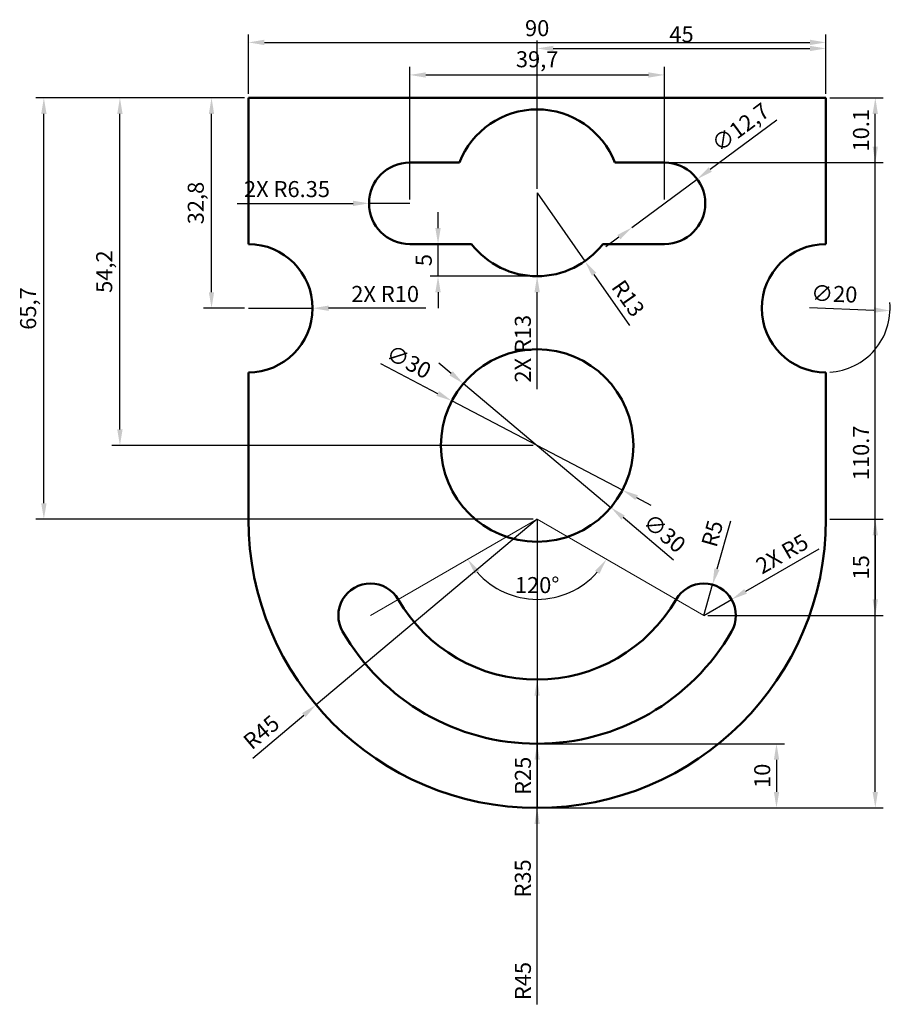
# Model space of a CAD drawing. Units: millimetres. Extents: x 2184 to 2320, y 1849 to 2003.
import ezdxf

# ---------------------------------------------------------------- set-up
doc = ezdxf.new("R2010")
doc.units = ezdxf.units.MM
for name, color, linetype, lineweight in [('M-CONS', 8, 'Continuous', 13), ('M-DIMS', 2, 'Continuous', 25), ('M-OUTL', 7, 'Continuous', 50)]:
    doc.layers.add(name, color=color, linetype=linetype, lineweight=lineweight)
doc.styles.get("Standard").update_dxf_attribs({"font": 'arial.ttf'})
doc.dimstyles.new('ISO-25', dxfattribs={"dimtxt": 2.5, "dimasz": 2.5, "dimexe": 1.25, "dimexo": 0.625, "dimtad": 1, "dimtxsty": 'Standard', "dimcen": 2.5, "dimadec": 0, "dimazin": 0, "dimtfac": 1, "dimtmove": 0, "dimatfit": 3, "dimfxl": 1, "dimarcsym": 0})

# ---------------------------------------------------------------- blocks, each defined once
blk = doc.blocks.new('*D1')
at = {"layer": 'Defpoints', "color": 0, "transparency": 16777216}
for p in [(2309.62, 1999.2), (2219.62, 1990.56), (2309.62, 1990.56)]:
    blk.add_point(p, dxfattribs=at)
at = {"layer": 'M-DIMS', "color": 0, "lineweight": -2, "transparency": 16777216}
for p, q in [((2219.62, 1991.18), (2219.62, 2000.45)), ((2309.62, 1991.18), (2309.62, 2000.45)), ((2222.12, 1999.2), (2307.12, 1999.2))]:
    blk.add_line(p, q, dxfattribs=at)
at = {"layer": 'M-DIMS', "color": 0, "transparency": 16777216}
for points in [[(2222.12, 1999.62), (2222.12, 1998.78), (2219.62, 1999.2)], [(2307.12, 1999.62), (2307.12, 1998.78), (2309.62, 1999.2)]]:
    blk.add_solid(points, dxfattribs=at)
at = {"layer": 'M-DIMS', "color": 0, "transparency": 16777216, "insert": (2264.62, 2001.1), "char_height": 2.5, "attachment_point": 5}
blk.add_mtext('90', dxfattribs=at)
blk = doc.blocks.new('*D2')
at = {"layer": 'Defpoints', "color": 0, "transparency": 16777216}
for p in [(2284.47, 1994.13), (2244.77, 1974.11), (2284.47, 1974.11)]:
    blk.add_point(p, dxfattribs=at)
at = {"layer": 'M-DIMS', "color": 0, "lineweight": -2, "transparency": 16777216}
for p, q in [((2244.77, 1974.73), (2244.77, 1995.38)), ((2247.27, 1994.13), (2281.97, 1994.13)), ((2284.47, 1974.73), (2284.47, 1995.38))]:
    blk.add_line(p, q, dxfattribs=at)
at = {"layer": 'M-DIMS', "color": 0, "transparency": 16777216}
for points in [[(2247.27, 1994.54), (2247.27, 1993.71), (2244.77, 1994.13)], [(2281.97, 1994.54), (2281.97, 1993.71), (2284.47, 1994.13)]]:
    blk.add_solid(points, dxfattribs=at)
at = {"layer": 'M-DIMS', "color": 0, "transparency": 16777216, "insert": (2264.62, 1996.25), "char_height": 2.5, "attachment_point": 5}
blk.add_mtext('39,7', dxfattribs=at)
blk = doc.blocks.new('*D3')
at = {"layer": 'Defpoints', "color": 0, "transparency": 16777216}
for p in [(2249.17, 1967.76), (2254.37, 1967.76), (2264.62, 1962.76)]:
    blk.add_point(p, dxfattribs=at)
at = {"layer": 'M-DIMS', "color": 0, "lineweight": -2, "transparency": 16777216}
for p, q in [((2249.17, 1970.26), (2249.17, 1972.76)), ((2253.75, 1967.76), (2247.92, 1967.76)), ((2249.17, 1962.76), (2249.17, 1967.76)), ((2263.99, 1962.76), (2247.92, 1962.76)), ((2249.17, 1960.26), (2249.17, 1957.76))]:
    blk.add_line(p, q, dxfattribs=at)
at = {"layer": 'M-DIMS', "color": 0, "transparency": 16777216}
for points in [[(2248.75, 1970.26), (2249.59, 1970.26), (2249.17, 1967.76)], [(2248.75, 1960.26), (2249.59, 1960.26), (2249.17, 1962.76)]]:
    blk.add_solid(points, dxfattribs=at)
at = {"layer": 'M-DIMS', "color": 0, "transparency": 16777216, "insert": (2247.27, 1965.26), "char_height": 2.5, "attachment_point": 5, "rotation": 90}
blk.add_mtext('5', dxfattribs=at)
blk = doc.blocks.new('*D4')
at = {"layer": 'Defpoints', "color": 0, "transparency": 16777216}
for p in [(2213.87, 1990.56), (2219.62, 1990.56), (2219.62, 1957.76)]:
    blk.add_point(p, dxfattribs=at)
at = {"layer": 'M-DIMS', "color": 0, "lineweight": -2, "transparency": 16777216}
for p, q in [((2218.99, 1990.56), (2212.62, 1990.56)), ((2213.87, 1960.26), (2213.87, 1988.06)), ((2218.99, 1957.76), (2212.62, 1957.76))]:
    blk.add_line(p, q, dxfattribs=at)
at = {"layer": 'M-DIMS', "color": 0, "transparency": 16777216}
for points in [[(2213.45, 1988.06), (2214.28, 1988.06), (2213.87, 1990.56)], [(2213.45, 1960.26), (2214.28, 1960.26), (2213.87, 1957.76)]]:
    blk.add_solid(points, dxfattribs=at)
at = {"layer": 'M-DIMS', "color": 0, "transparency": 16777216, "insert": (2211.74, 1974.16), "char_height": 2.5, "attachment_point": 5, "rotation": 90}
blk.add_mtext('32,8', dxfattribs=at)
blk = doc.blocks.new('*D5')
at = {"layer": 'Defpoints', "color": 0, "transparency": 16777216}
for p in [(2199.59, 1990.56), (2219.62, 1990.56), (2264.62, 1936.36)]:
    blk.add_point(p, dxfattribs=at)
at = {"layer": 'M-DIMS', "color": 0, "lineweight": -2, "transparency": 16777216}
for p, q in [((2218.99, 1990.56), (2198.34, 1990.56)), ((2199.59, 1938.86), (2199.59, 1988.06)), ((2263.99, 1936.36), (2198.34, 1936.36))]:
    blk.add_line(p, q, dxfattribs=at)
at = {"layer": 'M-DIMS', "color": 0, "transparency": 16777216}
for points in [[(2199.18, 1988.06), (2200.01, 1988.06), (2199.59, 1990.56)], [(2199.18, 1938.86), (2200.01, 1938.86), (2199.59, 1936.36)]]:
    blk.add_solid(points, dxfattribs=at)
at = {"layer": 'M-DIMS', "color": 0, "transparency": 16777216, "insert": (2197.47, 1963.46), "char_height": 2.5, "attachment_point": 5, "rotation": 90}
blk.add_mtext('54,2', dxfattribs=at)
blk = doc.blocks.new('*D6')
at = {"layer": 'Defpoints', "color": 0, "transparency": 16777216}
for p in [(2187.74, 1990.56), (2219.62, 1990.56), (2264.62, 1924.86)]:
    blk.add_point(p, dxfattribs=at)
at = {"layer": 'M-DIMS', "color": 0, "lineweight": -2, "transparency": 16777216}
for p, q in [((2218.99, 1990.56), (2186.49, 1990.56)), ((2187.74, 1927.36), (2187.74, 1988.06)), ((2263.99, 1924.86), (2186.49, 1924.86))]:
    blk.add_line(p, q, dxfattribs=at)
at = {"layer": 'M-DIMS', "color": 0, "transparency": 16777216}
for points in [[(2187.32, 1988.06), (2188.16, 1988.06), (2187.74, 1990.56)], [(2187.32, 1927.36), (2188.16, 1927.36), (2187.74, 1924.86)]]:
    blk.add_solid(points, dxfattribs=at)
at = {"layer": 'M-DIMS', "color": 0, "transparency": 16777216, "insert": (2185.61, 1957.71), "char_height": 2.5, "attachment_point": 5, "rotation": 90}
blk.add_mtext('65,7', dxfattribs=at)
blk = doc.blocks.new('*D7')
at = {"layer": 'Defpoints', "color": 0, "transparency": 16777216}
for p in [(2264.62, 1889.86), (2264.62, 1879.86), (2301.92, 1879.86)]:
    blk.add_point(p, dxfattribs=at)
at = {"layer": 'M-DIMS', "color": 0, "lineweight": -2, "transparency": 16777216}
for p, q in [((2265.24, 1889.86), (2303.17, 1889.86)), ((2301.92, 1887.36), (2301.92, 1882.36)), ((2265.24, 1879.86), (2303.17, 1879.86))]:
    blk.add_line(p, q, dxfattribs=at)
at = {"layer": 'M-DIMS', "color": 0, "transparency": 16777216}
for points in [[(2301.51, 1887.36), (2302.34, 1887.36), (2301.92, 1889.86)], [(2301.51, 1882.36), (2302.34, 1882.36), (2301.92, 1879.86)]]:
    blk.add_solid(points, dxfattribs=at)
at = {"layer": 'M-DIMS', "color": 0, "transparency": 16777216, "insert": (2300.02, 1884.86), "char_height": 2.5, "attachment_point": 5, "rotation": 90}
blk.add_mtext('10', dxfattribs=at)
blk = doc.blocks.new('*D8')
at = {"layer": 'Defpoints', "color": 0, "transparency": 16777216}
for p in [(2264.62, 1924.86), (2264.62, 1924.86), (2260.35, 1913.12), (2242.97, 1912.36), (2286.27, 1912.36)]:
    blk.add_point(p, dxfattribs=at)
at = {"layer": 'M-DIMS', "color": 0, "lineweight": -2, "transparency": 16777216}
blk.add_arc((2264.62, 1924.86), 12.49, 221.4867, 318.5133, dxfattribs=at)
at = {"layer": 'M-DIMS', "color": 0, "transparency": 16777216}
for points in [[(2254.92, 1916.34), (2255.6, 1916.82), (2253.8, 1918.61)], [(2273.64, 1916.82), (2274.31, 1916.34), (2275.43, 1918.61)]]:
    blk.add_solid(points, dxfattribs=at)
at = {"layer": 'M-DIMS', "color": 0, "transparency": 16777216, "insert": (2264.62, 1914.27), "char_height": 2.5, "attachment_point": 5}
blk.add_mtext('120°', dxfattribs=at)
blk = doc.blocks.new('*D9')
at = {"layer": 'Defpoints', "color": 0, "transparency": 16777216}
for p in [(2264.62, 1924.86), (2230.16, 1895.92)]:
    blk.add_point(p, dxfattribs=at)
at = {"layer": 'M-DIMS', "color": 0, "lineweight": -2, "transparency": 16777216}
for p, q in [((2264.62, 1924.86), (2230.16, 1895.92)), ((2220.29, 1887.63), (2228.24, 1894.31))]:
    blk.add_line(p, q, dxfattribs=at)
at = {"layer": 'M-DIMS', "color": 0, "transparency": 16777216}
blk.add_solid([(2227.97, 1894.63), (2228.51, 1893.99), (2230.16, 1895.92)], dxfattribs=at)
at = {"layer": 'M-DIMS', "color": 0, "transparency": 16777216, "insert": (2221.84, 1891.41), "char_height": 2.5, "attachment_point": 5, "rotation": 40.021}
blk.add_mtext('R45', dxfattribs=at)
blk = doc.blocks.new('*D10')
at = {"layer": 'Defpoints', "color": 0, "transparency": 16777216}
for p in [(2291.96, 1914.67), (2290.6, 1909.86)]:
    blk.add_point(p, dxfattribs=at)
at = {"layer": 'M-DIMS', "color": 0, "lineweight": -2, "transparency": 16777216}
for p, q in [((2294.77, 1924.58), (2292.64, 1917.07)), ((2290.6, 1909.86), (2291.96, 1914.67))]:
    blk.add_line(p, q, dxfattribs=at)
at = {"layer": 'M-DIMS', "color": 0, "transparency": 16777216}
blk.add_solid([(2292.24, 1917.19), (2293.04, 1916.96), (2291.96, 1914.67)], dxfattribs=at)
at = {"layer": 'M-DIMS', "color": 0, "transparency": 16777216, "insert": (2292.22, 1922.54), "char_height": 2.5, "attachment_point": 5, "rotation": 74.1736}
blk.add_mtext('R5', dxfattribs=at)
blk = doc.blocks.new('*D11')
at = {"layer": 'Defpoints', "color": 0, "transparency": 16777216}
for p in [(2264.62, 1975.76), (2272.06, 1965.09)]:
    blk.add_point(p, dxfattribs=at)
at = {"layer": 'M-DIMS', "color": 0, "lineweight": -2, "transparency": 16777216}
for p, q in [((2264.62, 1975.76), (2272.06, 1965.09)), ((2279.05, 1955.07), (2273.49, 1963.04))]:
    blk.add_line(p, q, dxfattribs=at)
at = {"layer": 'M-DIMS', "color": 0, "transparency": 16777216}
blk.add_solid([(2273.83, 1963.28), (2273.15, 1962.81), (2272.06, 1965.09)], dxfattribs=at)
at = {"layer": 'M-DIMS', "color": 0, "transparency": 16777216, "insert": (2278.54, 1959.12), "char_height": 2.5, "attachment_point": 5, "rotation": 304.9068}
blk.add_mtext('R13', dxfattribs=at)
blk = doc.blocks.new('*D12')
at = {"layer": 'Defpoints', "color": 0, "transparency": 16777216}
for p in [(2289.57, 1977.88), (2279.36, 1970.33)]:
    blk.add_point(p, dxfattribs=at)
at = {"layer": 'M-DIMS', "color": 0, "lineweight": -2, "transparency": 16777216}
for p, q in [((2302, 1987.09), (2291.58, 1979.37)), ((2279.36, 1970.33), (2289.57, 1977.88)), ((2277.35, 1968.84), (2275.34, 1967.35))]:
    blk.add_line(p, q, dxfattribs=at)
at = {"layer": 'M-DIMS', "color": 0, "transparency": 16777216}
for points in [[(2291.33, 1979.71), (2291.83, 1979.04), (2289.57, 1977.88)], [(2277.11, 1969.18), (2277.6, 1968.51), (2279.36, 1970.33)]]:
    blk.add_solid(points, dxfattribs=at)
at = {"layer": 'M-DIMS', "color": 0, "transparency": 16777216, "insert": (2296.5, 1985.72), "char_height": 2.5, "attachment_point": 5, "rotation": 36.5127}
blk.add_mtext('∅12,7', dxfattribs=at)
blk = doc.blocks.new('*D13')
at = {"layer": 'Defpoints', "color": 0, "transparency": 16777216}
for p in [(2299.62, 1958.13), (2319.61, 1957.38)]:
    blk.add_point(p, dxfattribs=at)
at = {"layer": 'M-DIMS', "color": 0, "lineweight": -2, "transparency": 16777216}
blk.add_line((2307.08, 1957.85), (2317.11, 1957.47), dxfattribs=at)
blk.add_arc((2309.62, 1957.76), 10, 273.581, 5.004, dxfattribs=at)
at = {"layer": 'M-DIMS', "color": 0, "transparency": 16777216}
blk.add_solid([(2317.13, 1957.89), (2317.1, 1957.06), (2319.61, 1957.38)], dxfattribs=at)
at = {"layer": 'M-DIMS', "color": 0, "transparency": 16777216, "insert": (2310.92, 1959.68), "char_height": 2.5, "attachment_point": 5, "rotation": 357.8421}
blk.add_mtext('∅20', dxfattribs=at)
blk = doc.blocks.new('*D14')
at = {"layer": 'Defpoints', "color": 0, "transparency": 16777216}
for p in [(2251.33, 1943.31), (2277.91, 1929.4)]:
    blk.add_point(p, dxfattribs=at)
at = {"layer": 'M-DIMS', "color": 0, "lineweight": -2, "transparency": 16777216}
for p, q in [((2240.21, 1949.13), (2249.11, 1944.47)), ((2277.91, 1929.4), (2251.33, 1943.31)), ((2280.12, 1928.24), (2282.34, 1927.08))]:
    blk.add_line(p, q, dxfattribs=at)
at = {"layer": 'M-DIMS', "color": 0, "transparency": 16777216}
for points in [[(2249.31, 1944.84), (2248.92, 1944.1), (2251.33, 1943.31)], [(2280.32, 1928.61), (2279.93, 1927.87), (2277.91, 1929.4)]]:
    blk.add_solid(points, dxfattribs=at)
at = {"layer": 'M-DIMS', "color": 0, "transparency": 16777216, "insert": (2244.47, 1949.12), "char_height": 2.5, "attachment_point": 5, "rotation": 332.3763}
blk.add_mtext('∅30', dxfattribs=at)
blk = doc.blocks.new('*D15')
at = {"layer": 'Defpoints', "color": 0, "transparency": 16777216}
for p in [(2309.62, 1990.56), (2317.32, 1990.56), (2264.62, 1879.86)]:
    blk.add_point(p, dxfattribs=at)
at = {"layer": 'M-DIMS', "color": 0, "lineweight": -2, "transparency": 16777216}
for p, q in [((2310.24, 1990.56), (2318.57, 1990.56)), ((2317.32, 1882.36), (2317.32, 1988.06)), ((2265.24, 1879.86), (2318.57, 1879.86))]:
    blk.add_line(p, q, dxfattribs=at)
at = {"layer": 'M-DIMS', "color": 0, "transparency": 16777216}
for points in [[(2316.9, 1988.06), (2317.73, 1988.06), (2317.32, 1990.56)], [(2316.9, 1882.36), (2317.73, 1882.36), (2317.32, 1879.86)]]:
    blk.add_solid(points, dxfattribs=at)
at = {"layer": 'M-DIMS', "color": 0, "transparency": 16777216, "insert": (2315.42, 1935.21), "char_height": 2.5, "attachment_point": 5, "rotation": 90}
blk.add_mtext('110.7', dxfattribs=at)
blk = doc.blocks.new('*D16')
at = {"layer": 'Defpoints', "color": 0, "transparency": 16777216}
for p in [(2309.62, 1998.26), (2309.62, 1990.56), (2264.62, 1975.76)]:
    blk.add_point(p, dxfattribs=at)
at = {"layer": 'M-DIMS', "color": 0, "lineweight": -2, "transparency": 16777216}
for p, q in [((2264.62, 1976.38), (2264.62, 1999.51)), ((2309.62, 1991.18), (2309.62, 1999.51)), ((2267.12, 1998.26), (2307.12, 1998.26))]:
    blk.add_line(p, q, dxfattribs=at)
at = {"layer": 'M-DIMS', "color": 0, "transparency": 16777216}
for points in [[(2267.12, 1998.67), (2267.12, 1997.84), (2264.62, 1998.26)], [(2307.12, 1998.67), (2307.12, 1997.84), (2309.62, 1998.26)]]:
    blk.add_solid(points, dxfattribs=at)
at = {"layer": 'M-DIMS', "color": 0, "transparency": 16777216, "insert": (2287.12, 2000.15), "char_height": 2.5, "attachment_point": 5}
blk.add_mtext('45', dxfattribs=at)
blk = doc.blocks.new('*D17')
at = {"layer": 'Defpoints', "color": 0, "transparency": 16777216}
for p in [(2309.62, 1990.56), (2317.32, 1990.56), (2276.74, 1980.46)]:
    blk.add_point(p, dxfattribs=at)
at = {"layer": 'M-DIMS', "color": 0, "lineweight": -2, "transparency": 16777216}
for p, q in [((2310.24, 1990.56), (2318.57, 1990.56)), ((2317.32, 1982.96), (2317.32, 1988.06)), ((2277.36, 1980.46), (2318.57, 1980.46))]:
    blk.add_line(p, q, dxfattribs=at)
at = {"layer": 'M-DIMS', "color": 0, "transparency": 16777216}
for points in [[(2316.9, 1988.06), (2317.73, 1988.06), (2317.32, 1990.56)], [(2316.9, 1982.96), (2317.73, 1982.96), (2317.32, 1980.46)]]:
    blk.add_solid(points, dxfattribs=at)
at = {"layer": 'M-DIMS', "color": 0, "transparency": 16777216, "insert": (2315.42, 1985.51), "char_height": 2.5, "attachment_point": 5, "rotation": 90}
blk.add_mtext('10.1', dxfattribs=at)
blk = doc.blocks.new('*D18')
at = {"layer": 'Defpoints', "color": 0, "transparency": 16777216}
for p in [(2309.62, 1924.86), (2290.6, 1909.86), (2317.32, 1909.86)]:
    blk.add_point(p, dxfattribs=at)
at = {"layer": 'M-DIMS', "color": 0, "lineweight": -2, "transparency": 16777216}
for p, q in [((2310.24, 1924.86), (2318.57, 1924.86)), ((2317.32, 1922.36), (2317.32, 1912.36)), ((2291.22, 1909.86), (2318.57, 1909.86))]:
    blk.add_line(p, q, dxfattribs=at)
at = {"layer": 'M-DIMS', "color": 0, "transparency": 16777216}
for points in [[(2316.9, 1922.36), (2317.73, 1922.36), (2317.32, 1924.86)], [(2316.9, 1912.36), (2317.73, 1912.36), (2317.32, 1909.86)]]:
    blk.add_solid(points, dxfattribs=at)
at = {"layer": 'M-DIMS', "color": 0, "transparency": 16777216, "insert": (2315.42, 1917.36), "char_height": 2.5, "attachment_point": 5, "rotation": 90}
blk.add_mtext('15', dxfattribs=at)
blk = doc.blocks.new('*D19')
at = {"layer": 'Defpoints', "color": 0, "transparency": 16777216}
for p in [(2253.13, 1946), (2276.11, 1926.71)]:
    blk.add_point(p, dxfattribs=at)
at = {"layer": 'M-DIMS', "color": 0, "lineweight": -2, "transparency": 16777216}
for p, q in [((2251.21, 1947.6), (2249.3, 1949.21)), ((2253.13, 1946), (2276.11, 1926.71)), ((2285.89, 1918.5), (2278.02, 1925.11))]:
    blk.add_line(p, q, dxfattribs=at)
at = {"layer": 'M-DIMS', "color": 0, "transparency": 16777216}
for points in [[(2251.48, 1947.92), (2250.94, 1947.29), (2253.13, 1946)], [(2278.29, 1925.43), (2277.76, 1924.79), (2276.11, 1926.71)]]:
    blk.add_solid(points, dxfattribs=at)
at = {"layer": 'M-DIMS', "color": 0, "transparency": 16777216, "insert": (2284.27, 1922.44), "char_height": 2.5, "attachment_point": 5, "rotation": 319.9995}
blk.add_mtext('∅30', dxfattribs=at)
blk = doc.blocks.new('*D20')
at = {"layer": 'Defpoints', "color": 0, "transparency": 16777216}
for p in [(2264.62, 1924.86), (2264.62, 1879.86)]:
    blk.add_point(p, dxfattribs=at)
at = {"layer": 'M-DIMS', "color": 0, "lineweight": -2, "transparency": 16777216}
for p, q in [((2264.62, 1924.86), (2264.62, 1879.86)), ((2264.62, 1849.23), (2264.62, 1877.36))]:
    blk.add_line(p, q, dxfattribs=at)
at = {"layer": 'M-DIMS', "color": 0, "transparency": 16777216}
blk.add_solid([(2264.2, 1877.36), (2265.03, 1877.36), (2264.62, 1879.86)], dxfattribs=at)
at = {"layer": 'M-DIMS', "color": 0, "transparency": 16777216, "insert": (2262.72, 1852.86), "char_height": 2.5, "attachment_point": 5, "rotation": 89.9997}
blk.add_mtext('R45', dxfattribs=at)
blk = doc.blocks.new('*D21')
at = {"layer": 'Defpoints', "color": 0, "transparency": 16777216}
for p in [(2264.62, 1924.86), (2264.62, 1889.86)]:
    blk.add_point(p, dxfattribs=at)
at = {"layer": 'M-DIMS', "color": 0, "lineweight": -2, "transparency": 16777216}
for p, q in [((2264.62, 1924.86), (2264.62, 1889.86)), ((2264.62, 1865.23), (2264.62, 1887.36))]:
    blk.add_line(p, q, dxfattribs=at)
at = {"layer": 'M-DIMS', "color": 0, "transparency": 16777216}
blk.add_solid([(2264.2, 1887.36), (2265.03, 1887.36), (2264.62, 1889.86)], dxfattribs=at)
at = {"layer": 'M-DIMS', "color": 0, "transparency": 16777216, "insert": (2262.71, 1868.86), "char_height": 2.5, "attachment_point": 5, "rotation": 89.9996}
blk.add_mtext('R35', dxfattribs=at)
blk = doc.blocks.new('*D22')
at = {"layer": 'Defpoints', "color": 0, "transparency": 16777216}
for p in [(2264.62, 1924.86), (2264.62, 1899.86)]:
    blk.add_point(p, dxfattribs=at)
at = {"layer": 'M-DIMS', "color": 0, "lineweight": -2, "transparency": 16777216}
for p, q in [((2264.62, 1924.86), (2264.62, 1899.86)), ((2264.62, 1881.23), (2264.62, 1897.36))]:
    blk.add_line(p, q, dxfattribs=at)
at = {"layer": 'M-DIMS', "color": 0, "transparency": 16777216}
blk.add_solid([(2264.2, 1897.36), (2265.03, 1897.36), (2264.62, 1899.86)], dxfattribs=at)
at = {"layer": 'M-DIMS', "color": 0, "transparency": 16777216, "insert": (2262.72, 1884.86), "char_height": 2.5, "attachment_point": 5, "rotation": 89.9995}
blk.add_mtext('R25', dxfattribs=at)
blk = doc.blocks.new('*D23')
at = {"layer": 'Defpoints', "color": 0, "transparency": 16777216}
for p in [(2264.62, 1975.76), (2264.62, 1962.76)]:
    blk.add_point(p, dxfattribs=at)
at = {"layer": 'M-DIMS', "color": 0, "lineweight": -2, "transparency": 16777216}
for p, q in [((2264.62, 1975.76), (2264.62, 1962.76)), ((2264.62, 1945.12), (2264.62, 1960.26))]:
    blk.add_line(p, q, dxfattribs=at)
at = {"layer": 'M-DIMS', "color": 0, "transparency": 16777216}
blk.add_solid([(2264.2, 1960.26), (2265.03, 1960.26), (2264.62, 1962.76)], dxfattribs=at)
at = {"layer": 'M-DIMS', "color": 0, "transparency": 16777216, "insert": (2262.71, 1951.44), "char_height": 2.5, "attachment_point": 5, "rotation": 89.999}
blk.add_mtext('2X R13', dxfattribs=at)
blk = doc.blocks.new('*D24')
at = {"layer": 'Defpoints', "color": 0, "transparency": 16777216}
for p in [(2219.62, 1957.76), (2229.62, 1957.76)]:
    blk.add_point(p, dxfattribs=at)
at = {"layer": 'M-DIMS', "color": 0, "lineweight": -2, "transparency": 16777216}
for p, q in [((2219.62, 1957.76), (2229.62, 1957.76)), ((2247.25, 1957.76), (2232.12, 1957.76))]:
    blk.add_line(p, q, dxfattribs=at)
at = {"layer": 'M-DIMS', "color": 0, "transparency": 16777216}
blk.add_solid([(2232.12, 1958.17), (2232.12, 1957.34), (2229.62, 1957.76)], dxfattribs=at)
at = {"layer": 'M-DIMS', "color": 0, "transparency": 16777216, "insert": (2240.93, 1959.66), "char_height": 2.5, "attachment_point": 5, "rotation": 359.9996}
blk.add_mtext('2X R10', dxfattribs=at)
blk = doc.blocks.new('*D25')
at = {"layer": 'Defpoints', "color": 0, "transparency": 16777216}
for p in [(2238.42, 1974.11), (2244.77, 1974.11)]:
    blk.add_point(p, dxfattribs=at)
at = {"layer": 'M-DIMS', "color": 0, "lineweight": -2, "transparency": 16777216}
for p, q in [((2217.85, 1974.11), (2235.92, 1974.11)), ((2244.77, 1974.11), (2238.42, 1974.11))]:
    blk.add_line(p, q, dxfattribs=at)
at = {"layer": 'M-DIMS', "color": 0, "transparency": 16777216}
blk.add_solid([(2235.92, 1974.52), (2235.92, 1973.69), (2238.42, 1974.11)], dxfattribs=at)
at = {"layer": 'M-DIMS', "color": 0, "transparency": 16777216, "insert": (2225.63, 1976.01), "char_height": 2.5, "attachment_point": 5, "rotation": 0.0006}
blk.add_mtext('2X R6.35', dxfattribs=at)
blk = doc.blocks.new('*D26')
at = {"layer": 'Defpoints', "color": 0, "transparency": 16777216}
for p in [(2294.93, 1912.36), (2290.6, 1909.86)]:
    blk.add_point(p, dxfattribs=at)
at = {"layer": 'M-DIMS', "color": 0, "lineweight": -2, "transparency": 16777216}
for p, q in [((2308.54, 1920.21), (2297.09, 1913.61)), ((2290.6, 1909.86), (2294.93, 1912.36))]:
    blk.add_line(p, q, dxfattribs=at)
at = {"layer": 'M-DIMS', "color": 0, "transparency": 16777216}
blk.add_solid([(2296.88, 1913.97), (2297.3, 1913.25), (2294.93, 1912.36)], dxfattribs=at)
at = {"layer": 'M-DIMS', "color": 0, "transparency": 16777216, "insert": (2302.95, 1919.18), "char_height": 2.5, "attachment_point": 5, "rotation": 30}
blk.add_mtext('2X R5', dxfattribs=at)

msp = doc.modelspace()

# ---------------------------------------------------------------- linework, layer by layer
at = {"layer": 'M-CONS'}
for p, q in [((2219.617, 1990.556), (2219.617, 1967.756)), ((2219.617, 1990.556), (2219.617, 1967.756)), ((2264.617, 1990.556), (2244.767, 1990.556)), ((2264.617, 1990.556), (2284.467, 1990.556)), ((2309.617, 1990.556), (2309.617, 1967.756)), ((2309.617, 1990.556), (2309.617, 1967.756)), ((2219.617, 1947.756), (2219.617, 1936.356)), ((2309.617, 1947.756), (2309.617, 1936.356)), ((2264.617, 1924.856), (2242.967, 1912.356)), ((2264.617, 1924.856), (2286.268, 1912.356)), ((2242.967, 1912.356), (2238.636, 1909.856)), ((2286.268, 1912.356), (2290.598, 1909.856))]:
    msp.add_line(p, q, dxfattribs=at)
at = {"layer": 'M-OUTL'}
for p, q in [((2219.617, 1990.556), (2309.617, 1990.556)), ((2219.617, 1990.556), (2219.617, 1967.756)), ((2309.617, 1990.556), (2309.617, 1967.756)), ((2244.767, 1980.456), (2252.497, 1980.456)), ((2276.738, 1980.456), (2284.467, 1980.456)), ((2244.767, 1967.756), (2254.37, 1967.756)), ((2274.864, 1967.756), (2284.467, 1967.756)), ((2219.617, 1947.756), (2219.617, 1924.856)), ((2309.617, 1947.756), (2309.617, 1924.856))]:
    msp.add_line(p, q, dxfattribs=at)
msp.add_circle((2264.617, 1936.356), 15, dxfattribs=at)
for centre, radius, start, end in [((2264.617, 1975.756), 13, 21.19471, 158.80529), ((2244.767, 1974.106), 6.35, 90, 270), ((2284.467, 1974.106), 6.35, 270, 90), ((2219.617, 1957.756), 10, 270, 90), ((2264.617, 1975.756), 13, 217.97987, 322.02013), ((2309.617, 1957.756), 10, 90, 270), ((2264.617, 1924.856), 45, 180, 0), ((2238.636, 1909.856), 5, 30, 210), ((2290.598, 1909.856), 5, 330, 150), ((2264.617, 1924.856), 25, 210, 330), ((2264.617, 1924.856), 35, 210, 330)]:
    msp.add_arc(centre, radius, start, end, dxfattribs=at)

# ---------------------------------------------------------------- dimensions: what is measured, and where the dimension line sits
at = {"layer": 'M-DIMS'}
for base, p1, p2, override, picture, middle in [((2309.617, 1999.201), (2219.617, 1990.556), (2309.617, 1990.556), {"dimclrd": 0, "dimclre": 0, "dimclrt": 0}, '*D1', (2264.617, 2001.102)), ((2309.617, 1998.256), (2264.617, 1975.756), (2309.617, 1990.556), {"dimdec": 0, "dimlfac": 1, "dimrnd": 0, "dimzin": 0, "dimdsep": 46, "dimlunit": 2}, '*D16', (2287.117, 2000.152)), ((2284.467, 1994.125), (2244.767, 1974.106), (2284.467, 1974.106), {"dimclrd": 0, "dimclre": 0, "dimclrt": 0}, '*D2', (2264.617, 1996.253))]:
    dim = msp.add_linear_dim(base=base, p1=p1, p2=p2, dimstyle='ISO-25', override=override, dxfattribs=at)
    dim.commit()
    dim.dimension.update_dxf_attribs({"geometry": picture, "text_midpoint": middle})
for base, p1, p2, override, picture, middle in [((2187.741, 1990.556), (2264.617, 1924.856), (2219.617, 1990.556), {"dimclrd": 0, "dimclre": 0, "dimclrt": 0}, '*D6', (2185.614, 1957.706)), ((2199.595, 1990.556), (2264.617, 1936.356), (2219.617, 1990.556), {"dimclrd": 0, "dimclre": 0, "dimclrt": 0}, '*D5', (2197.468, 1963.456)), ((2213.868, 1990.556), (2219.617, 1957.756), (2219.617, 1990.556), {"dimclrd": 0, "dimclre": 0, "dimclrt": 0}, '*D4', (2211.74, 1974.156)), ((2317.317, 1990.556), (2264.617, 1879.856), (2309.617, 1990.556), {"dimdec": 1, "dimlfac": 1, "dimrnd": 0, "dimzin": 0, "dimdsep": 46, "dimlunit": 2}, '*D15', (2315.416, 1935.206)), ((2317.317, 1990.556), (2276.738, 1980.456), (2309.617, 1990.556), {"dimdec": 1, "dimlfac": 1, "dimrnd": 0, "dimzin": 0, "dimdsep": 46, "dimlunit": 2}, '*D17', (2315.416, 1985.506)), ((2249.17, 1967.756), (2264.617, 1962.756), (2254.37, 1967.756), {"dimclrd": 0, "dimclre": 0, "dimclrt": 0}, '*D3', (2247.273, 1965.256)), ((2317.317, 1909.856), (2309.617, 1924.856), (2290.598, 1909.856), {"dimdec": 0, "dimlfac": 1, "dimrnd": 0, "dimzin": 0, "dimdsep": 46, "dimlunit": 2}, '*D18', (2315.416, 1917.356)), ((2301.925, 1879.856), (2264.617, 1889.856), (2264.617, 1879.856), {"dimclrd": 0, "dimclre": 0, "dimclrt": 0}, '*D7', (2300.023, 1884.856))]:
    dim = msp.add_linear_dim(base=base, p1=p1, p2=p2, angle=90, dimstyle='ISO-25', override=override, dxfattribs=at)
    dim.commit()
    dim.dimension.update_dxf_attribs({"geometry": picture, "text_midpoint": middle})
for p1, p2, picture, middle in [((2279.364, 1970.328), (2289.571, 1977.884), '*D12', (2296.504, 1985.715)), ((2277.907, 1929.401), (2251.327, 1943.311), '*D14', (2244.47, 1949.125))]:
    dim = msp.add_diameter_dim_2p(p1=p1, p2=p2, dimstyle='ISO-25', override={"dimclrd": 0, "dimclre": 0, "dimclrt": 0}, dxfattribs=at)
    dim.commit()
    dim.dimension.update_dxf_attribs({"geometry": picture, "text_midpoint": middle})
for center, mpoint, override, picture, middle in [((2244.767, 1974.106), (2238.417, 1974.106), {"dimdec": 2, "dimlfac": 1, "dimrnd": 0, "dimzin": 0, "dimdsep": 46, "dimlunit": 2}, '*D25', (2225.632, 1976.008)), ((2264.617, 1975.756), (2264.617, 1962.756), {"dimdec": 0, "dimlfac": 1, "dimrnd": 0, "dimzin": 0, "dimdsep": 46, "dimlunit": 2}, '*D23', (2262.715, 1951.437)), ((2219.617, 1957.756), (2229.617, 1957.756), {"dimdec": 0, "dimlfac": 1, "dimrnd": 0, "dimzin": 0, "dimdsep": 46, "dimlunit": 2}, '*D24', (2240.932, 1959.657)), ((2290.598, 1909.856), (2294.928, 1912.356), {"dimdec": 0, "dimlfac": 1, "dimrnd": 0, "dimzin": 0, "dimdsep": 46, "dimlunit": 2}, '*D26', (2302.947, 1919.181))]:
    dim = msp.add_radius_dim(center=center, mpoint=mpoint, text='2X <>', dimstyle='ISO-25', override=override, dxfattribs=at)
    dim.commit()
    dim.dimension.update_dxf_attribs({"geometry": picture, "text_midpoint": middle})
for center, mpoint, picture, middle in [((2264.617, 1975.756), (2272.056, 1965.095), '*D11', (2278.545, 1959.121)), ((2290.598, 1909.856), (2291.962, 1914.667), '*D10', (2292.224, 1922.544))]:
    dim = msp.add_radius_dim(center=center, mpoint=mpoint, dimstyle='ISO-25', override={"dimclrd": 0, "dimclre": 0, "dimclrt": 0}, dxfattribs=at)
    dim.commit()
    dim.dimension.update_dxf_attribs({"geometry": picture, "text_midpoint": middle})
for p1, p2, override, picture, middle in [((2299.624, 1958.133), (2319.61, 1957.38), {"dimclrd": 0, "dimclre": 0, "dimclrt": 0}, '*D13', (2310.845, 1957.71)), ((2253.127, 1945.998), (2276.108, 1926.714), {"dimdec": 0, "dimlfac": 1, "dimrnd": 0, "dimzin": 0, "dimdsep": 46, "dimlunit": 2}, '*D19', (2283.002, 1920.929))]:
    dim = msp.add_diameter_dim_2p(p1=p1, p2=p2, dimstyle='ISO-25', override=override, dxfattribs=at)
    dim.commit()
    dim.dimension.update_dxf_attribs({"geometry": picture, "text_midpoint": middle, "dimtype": 163})
for mpoint, override, picture, middle in [((2230.156, 1895.918), {"dimclrd": 0, "dimclre": 0, "dimclrt": 0}, '*D9', (2223.061, 1889.96)), ((2264.617, 1889.856), {"dimdec": 0, "dimlfac": 1, "dimrnd": 0, "dimzin": 0, "dimdsep": 46, "dimlunit": 2}, '*D21', (2264.617, 1868.856)), ((2264.617, 1899.856), {"dimdec": 0, "dimlfac": 1, "dimrnd": 0, "dimzin": 0, "dimdsep": 46, "dimlunit": 2}, '*D22', (2264.617, 1884.856)), ((2264.617, 1879.856), {"dimdec": 0, "dimlfac": 1, "dimrnd": 0, "dimzin": 0, "dimdsep": 46, "dimlunit": 2}, '*D20', (2264.617, 1852.856))]:
    dim = msp.add_radius_dim(center=(2264.617, 1924.856), mpoint=mpoint, dimstyle='ISO-25', override=override, dxfattribs=at)
    dim.commit()
    dim.dimension.update_dxf_attribs({"geometry": picture, "text_midpoint": middle, "dimtype": 164})
dim = msp.add_angular_dim_2l(base=(2260.345, 1913.118), line1=((2264.617, 1924.856), (2286.268, 1912.356)), line2=((2264.617, 1924.856), (2242.967, 1912.356)), dimstyle='ISO-25', override={"dimclrd": 0, "dimclre": 0, "dimclrt": 0}, dxfattribs=at)
dim.commit()
dim.dimension.update_dxf_attribs({"geometry": '*D8', "text_midpoint": (2264.617, 1914.267)})

doc.saveas('drawing.dxf')
